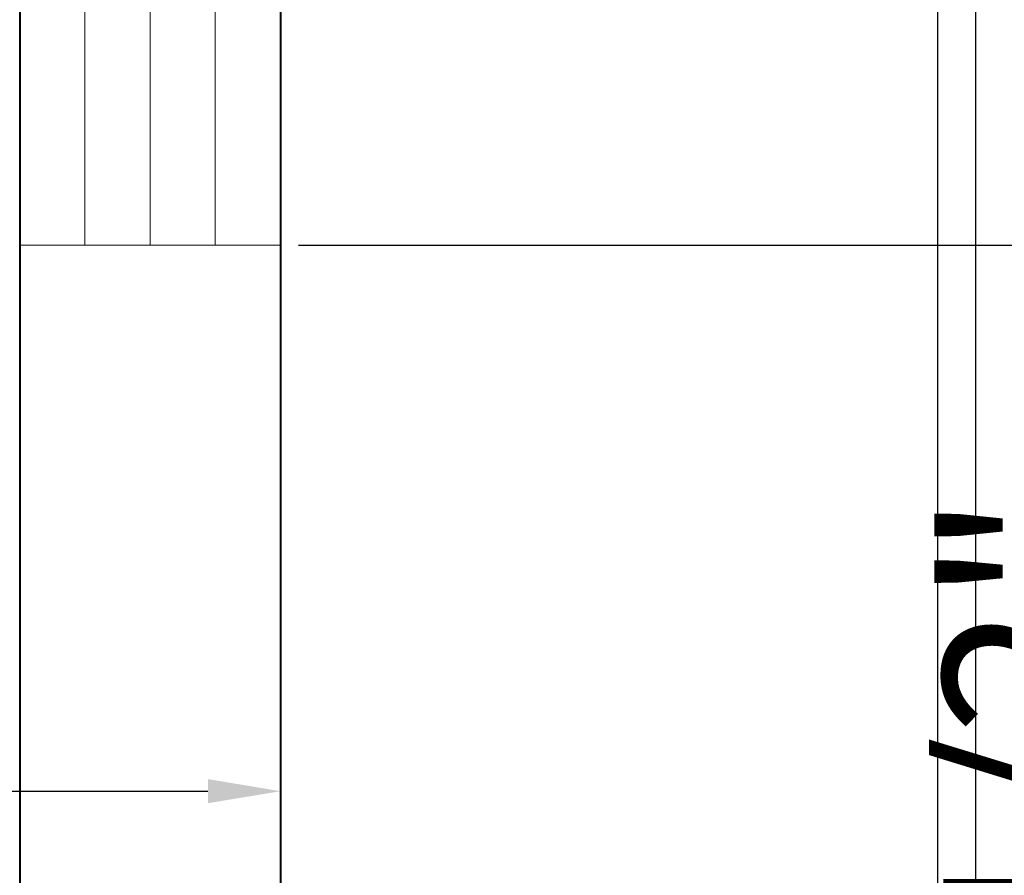
# Model space of a CAD drawing. Units: inches. Extents: x 459864 to 460310, y 324185 to 324787.
# Tile 107 of 112: x 460238 to 460272, y 324311 to 324341. Entities that reach past the tile are written whole.
import ezdxf

# ---------------------------------------------------------------- set-up
doc = ezdxf.new("R2010")
doc.units = ezdxf.units.IN
for name, color, linetype, lineweight in [('A-ANNO-DIMS', 2, 'Continuous', 18), ('A-GLAZ', 4, 'Continuous', 18), ('A-WALL', 7, 'Continuous', 40), ('C-PROP', 7, 'Continuous', 30)]:
    doc.layers.add(name, color=color, linetype=linetype, lineweight=lineweight)
doc.styles.get("Standard").update_dxf_attribs({"font": 'arial.ttf'})
doc.dimstyles.new('ISO-25', dxfattribs={"dimtxt": 6, "dimasz": 2.5, "dimexe": 1.25, "dimexo": 0.625, "dimtad": 1, "dimdec": 1, "dimlunit": 3, "dimtxsty": 'Standard', "dimcen": 2.5, "dimadec": 0, "dimazin": 0, "dimtfac": 1, "dimtdec": 1, "dimtmove": 0, "dimatfit": 3, "dimfxl": 1, "dimarcsym": 0})

# ---------------------------------------------------------------- blocks, each defined once
blk = doc.blocks.new('Window - Wood Frame 36 in. Wide plan')
for p, q in [((0, 6), (0, 0)), ((36, 6), (36, 0)), ((0, 4.5), (36, 4.5)), ((0, 3), (36, 3)), ((0, 1.5), (36, 1.5))]:
    blk.add_line(p, q)
blk = doc.blocks.new('*D21')
at = {"layer": 'A-ANNO-DIMS', "color": 0, "lineweight": -2, "transparency": 16777216}
for p, q in [((460247.74, 324715.483), (460309.58, 324715.483)), ((460308.33, 324712.983), (460308.33, 324285.983)), ((460247.74, 324283.483), (460309.58, 324283.483))]:
    blk.add_line(p, q, dxfattribs=at)
at = {"layer": 'A-ANNO-DIMS', "color": 0, "transparency": 16777216}
for points in [[(460307.914, 324712.983), (460308.747, 324712.983), (460308.33, 324715.483)], [(460307.914, 324285.983), (460308.747, 324285.983), (460308.33, 324283.483)]]:
    blk.add_solid(points, dxfattribs=at)
at = {"layer": 'Defpoints', "color": 0, "transparency": 16777216}
for p in [(460247.115, 324715.483), (460247.115, 324283.483), (460308.33, 324283.483)]:
    blk.add_point(p, dxfattribs=at)
at = {"layer": 'A-ANNO-DIMS', "color": 0, "transparency": 16777216, "insert": (460304.64, 324499.483), "char_height": 6, "attachment_point": 5, "rotation": 90}
blk.add_mtext("36'", dxfattribs=at)
blk = doc.blocks.new('*D62')
at = {"layer": 'A-ANNO-DIMS', "color": 0, "lineweight": -2, "transparency": 16777216}
for p, q in [((460247.74, 324332.739), (460278.765, 324332.739)), ((460277.515, 324330.239), (460277.515, 324285.983)), ((460247.74, 324283.483), (460278.765, 324283.483))]:
    blk.add_line(p, q, dxfattribs=at)
at = {"layer": 'A-ANNO-DIMS', "color": 0, "transparency": 16777216}
for points in [[(460277.098, 324330.239), (460277.932, 324330.239), (460277.515, 324332.739)], [(460277.098, 324285.983), (460277.932, 324285.983), (460277.515, 324283.483)]]:
    blk.add_solid(points, dxfattribs=at)
at = {"layer": 'Defpoints', "color": 0, "transparency": 16777216}
for p in [(460247.115, 324332.739), (460247.115, 324283.483), (460277.515, 324283.483)]:
    blk.add_point(p, dxfattribs=at)
at = {"layer": 'A-ANNO-DIMS', "color": 0, "transparency": 16777216, "insert": (460273.788, 324308.111), "char_height": 6, "attachment_point": 5, "rotation": 90}
blk.add_mtext('4\'-1 1/2"', dxfattribs=at)
blk = doc.blocks.new('*D67')
at = {"layer": 'A-ANNO-DIMS', "color": 0, "lineweight": -2, "transparency": 16777216}
for p, q in [((460208.115, 324284.108), (460208.115, 324315.133)), ((460247.115, 324284.108), (460247.115, 324315.133)), ((460210.615, 324313.883), (460244.615, 324313.883))]:
    blk.add_line(p, q, dxfattribs=at)
at = {"layer": 'A-ANNO-DIMS', "color": 0, "transparency": 16777216}
for points in [[(460210.615, 324314.3), (460210.615, 324313.467), (460208.115, 324313.883)], [(460244.615, 324314.3), (460244.615, 324313.467), (460247.115, 324313.883)]]:
    blk.add_solid(points, dxfattribs=at)
at = {"layer": 'Defpoints', "color": 0, "transparency": 16777216}
for p in [(460247.115, 324313.883), (460208.115, 324283.483), (460247.115, 324283.483)]:
    blk.add_point(p, dxfattribs=at)
at = {"layer": 'A-ANNO-DIMS', "color": 0, "transparency": 16777216, "insert": (460227.615, 324317.574), "char_height": 6, "attachment_point": 5}
blk.add_mtext('3\'-3"', dxfattribs=at)

msp = doc.modelspace()

# ---------------------------------------------------------------- linework, layer by layer
at = {"layer": 'A-WALL'}
for p, q in [((460247.115, 324470.983), (460247.115, 324283.483)), ((460238.115, 324466.483), (460238.115, 324292.483))]:
    msp.add_line(p, q, dxfattribs=at)
at = {"layer": 'C-PROP'}
for p, q in [((460269.804, 324466.483), (460269.804, 324199.483)), ((460271.115, 324466.483), (460271.115, 324194.947))]:
    msp.add_line(p, q, dxfattribs=at)

# ---------------------------------------------------------------- block references
at = {"layer": 'A-GLAZ', "xscale": 1.5, "yscale": 1.5, "zscale": 1.5, "rotation": 90}
msp.add_blockref('Window - Wood Frame 36 in. Wide plan', (460247.115, 324332.739), dxfattribs=at)

# ---------------------------------------------------------------- dimensions: what is measured, and where the dimension line sits
at = {"layer": 'A-ANNO-DIMS'}
for base, p1, angle, override, picture, middle in [((460308.33, 324283.483), (460247.115, 324715.483), 90, {"dimclrd": 0, "dimclre": 0, "dimclrt": 0}, '*D21', (460304.64, 324499.483)), ((460277.515, 324283.483), (460247.115, 324332.739), 270, {"dimdec": 1, "dimlfac": 1, "dimrnd": 0, "dimzin": 1, "dimdsep": 46, "dimlunit": 4, "dimfrac": 2}, '*D62', (460273.788, 324308.111))]:
    dim = msp.add_linear_dim(base=base, p1=p1, p2=(460247.115, 324283.483), angle=angle, dimstyle='ISO-25', override=override, dxfattribs=at)
    dim.commit()
    dim.dimension.update_dxf_attribs({"geometry": picture, "text_midpoint": middle})
dim = msp.add_linear_dim(base=(460247.115, 324313.883), p1=(460208.115, 324283.483), p2=(460247.115, 324283.483), dimstyle='ISO-25', override={"dimdec": 1, "dimlfac": 1, "dimrnd": 0, "dimzin": 1, "dimdsep": 46, "dimlunit": 4, "dimfrac": 2}, dxfattribs=at)
dim.commit()
dim.dimension.update_dxf_attribs({"geometry": '*D67', "text_midpoint": (460227.615, 324317.574)})

doc.saveas('drawing.dxf')
